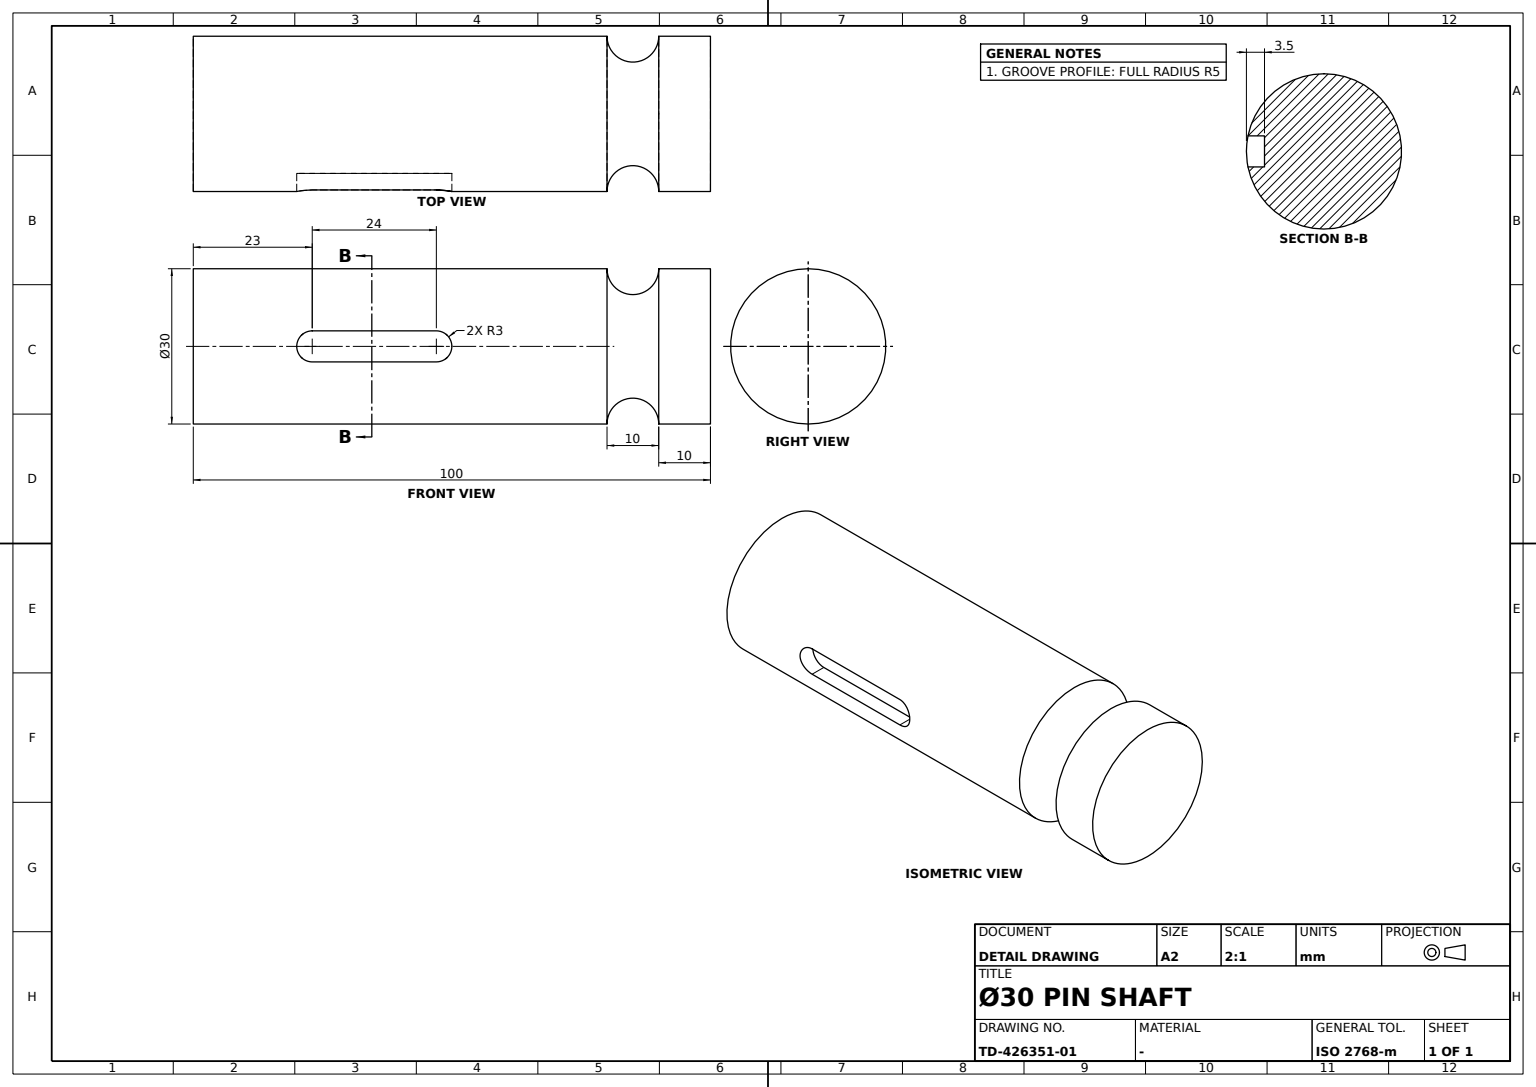
CATIA V5 part; units mm, degrees
sketch "Sketch1" plane through (0, 0, 0) normal (0, 1, 0) x (-1, 0, 0)
  circle A0 centre (0, 0) radius 15
  dimension "radius A0" = 15
extrude "Pad1" add sketch "Sketch1" along normal blind 100
ref_plane "Plane1" through (15, 0, 0) normal (1, 0, 0) x (0, 1, 0)
sketch "Sketch2" plane through (15, 0, 0) normal (1, 0, 0) x (0, 1, 0)
  arc A0 (23, 3) -> (23, -3) centre (23, 0) ccw
  arc A1 (47, -3) -> (47, 3) centre (47, 0) ccw
  line L0 (23, 3) -> (47, 3)
  line L1 (23, -3) -> (47, -3)
  dimension "radius A0" = 3
  dimension "radius A1" = 3
  constraint tangency L0 A0
  constraint tangency L0 A1
  constraint tangency L1 A0
  constraint tangency L1 A1
extrude "Pocket1" cut sketch "Sketch2" against normal blind 3.5
sketch "Sketch3" plane through (0, 0, 0) normal (1, 0, 0) x (0, 1, 0)
  point P0 (100, 15)
  circle A0 centre (85, 15) radius 5
  point P1 (85, 15)
  dimension "radius A0" = 5
  dimension "distance P1 P0" = 15
revolve "Groove1" cut sketch "Sketch3" angle 360 about axis through (0, 0, 0) along (0, 1, 0)
